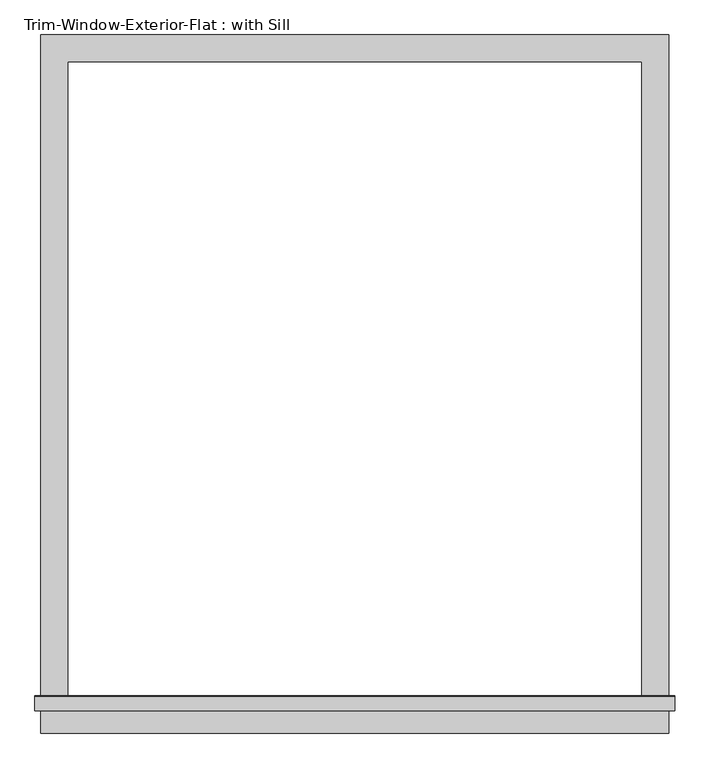
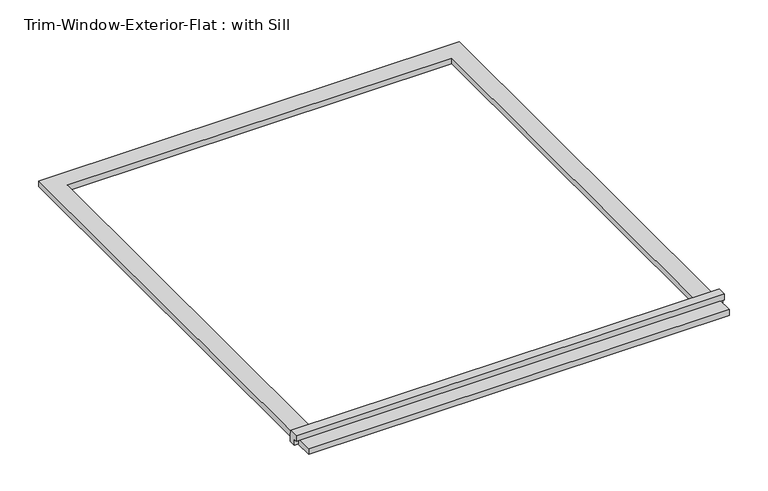
"""IFC4 building model written with IfcOpenShell, lengths in millimetres: proxy geometry, Trim-Window-Exterior-Flat : with Sill."""

from ifc_helpers import new_model, si_unit, frame, origin, origin_with_axes, place, context, project, spatial, polyline, outline, extrude, source, transform, mapped, element, save


def trim_window_exterior_flat_with_sill_fda35bc9(model_context):
    return source(origin(), model_context, "Body", "SweptSolid", [
        extrude(outline(polyline([(666.75, -1368.3823709), (666.75, -1425.5323709), (-666.75, -1425.5323709), (-666.75, -1368.3823709), (666.75, -1368.3823709)])), origin_with_axes(), (0.0, 0.0, 1.0), 19.05),
        extrude(outline(polyline([(-1377.95, 38.1), (-1348.6580645, 38.1), (-1346.2, 19.05), (-1346.2, 0.0), (-1368.3823709, 0.0), (-1368.3823709, 19.05), (-1377.95, 19.05), (-1377.95, 38.1)])), frame((-679.45, 0.0, 0.0), z_axis=(1.0, 0.0, 0.0), x_axis=(0.0, 1.0, 0.0)), (0.0, 0.0, 1.0), 1358.9),
        extrude(outline(polyline([(-666.75, 57.15), (666.75, 57.15), (666.75, -1346.2), (609.6, -1346.2), (609.6, 0.0), (-609.6, 0.0), (-609.6, -1346.2), (-666.75, -1346.2), (-666.75, 57.15)])), origin_with_axes(), (0.0, 0.0, 1.0), 19.05),
    ])


if __name__ == "__main__":
    model = new_model("IFC4")
    model_context = context("Model", 3, world=origin())
    ifc_project = project(units=[si_unit("LENGTHUNIT", "METRE", prefix="MILLI")], contexts=[model_context])
    site = spatial("IfcSite", under=ifc_project)
    building = spatial("IfcBuilding", under=site)
    placement = place(None, origin())
    trim_window_exterior_flat_with_sill_shape = trim_window_exterior_flat_with_sill_fda35bc9(model_context)
    element("IfcBuildingElementProxy", 1, Name="Trim-Window-Exterior-Flat : with Sill", ObjectType="Trim-Window-Exterior-Flat : with Sill", at=placement, inside=building, context=model_context, shape_type="MappedRepresentation", body=[
        mapped(trim_window_exterior_flat_with_sill_shape, transform((0.0, 0.0, 0.0), x_axis=(1.0, 0.0, 0.0), y_axis=(0.0, 1.0, 0.0), z_axis=(0.0, 0.0, 1.0))),
    ])
    save(model, "model.ifc")

# Revit data of these elements
# Type "Trim-Window-Exterior-Flat : with Sill"
#   Trim Width = 0' - 2 1/4"
#   Trim Thickness_Picture Frame = 0' - 1 1/4"
#   Trim Thickness_with Sill = 0' - 0 3/4"
#   Sill Thickness = 0' - 1 1/4"
#   Opening Width [instance default] = 2' - 0"
#   Opening Height [instance default] = 3' - 0"
#   Default Elevation = 4' - 0"
#   Sill = yes
#   Picture Frame = no
#   Trim Material [instance default] = none
# Element 1 (IfcBuildingElementProxy, "Trim-Window-Exterior-Flat : with Sill")
#   Opening Width = 4' - 0"
#   Opening Height = 4' - 5"
#   Trim Material = Clad - White
#   Materials on its faces: "Clad - White"
# Materials
#   "Clad - White": class "Wood", colour RGB 242 242 238, transparency 0, Cost = 0
